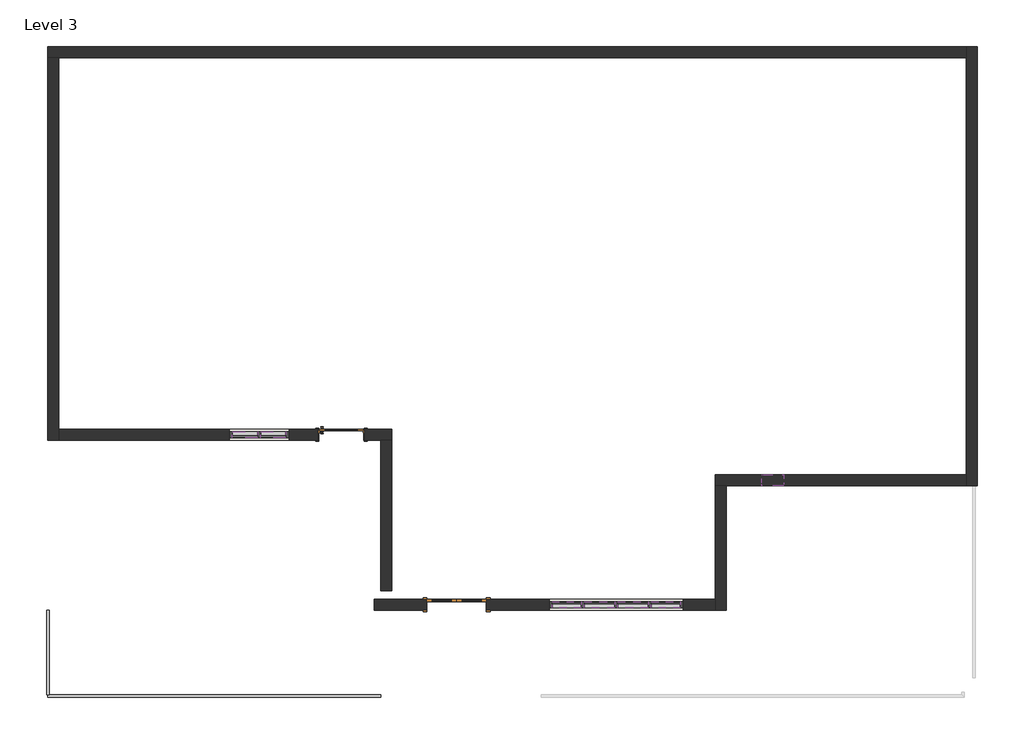
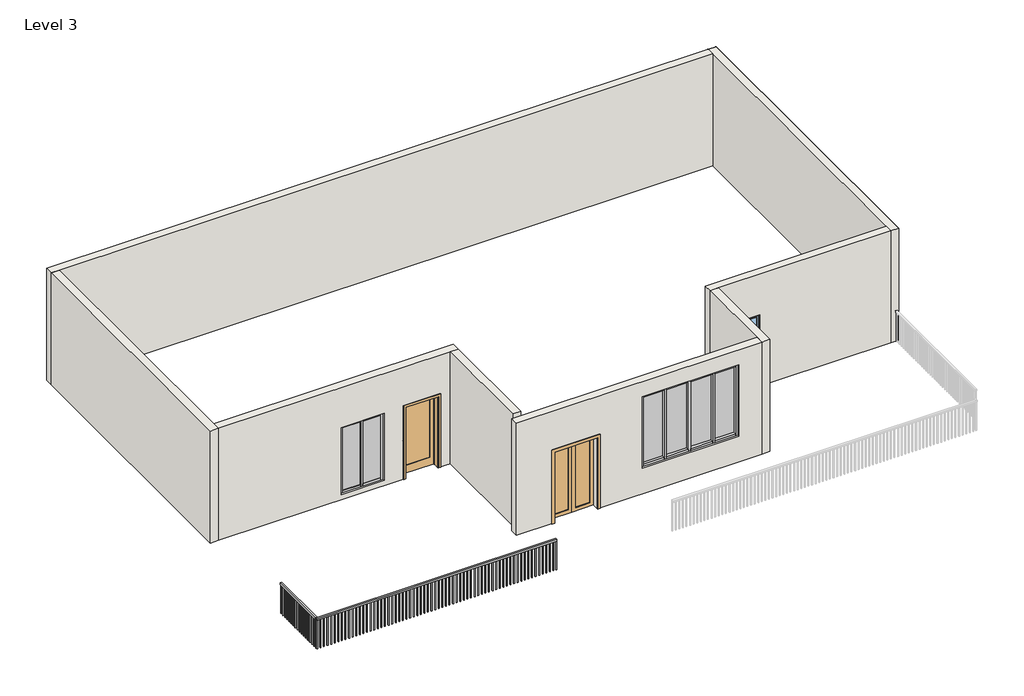
# One storey, part 1 of 2: 20 members, 8 walls, 6 plates, 2 doors, 2 railings, 1 window.
"""IFC4 building model written with IfcOpenShell, lengths in millimetres."""

from ifc_helpers import new_model, si_unit, frame, origin, place, context, project, spatial, polyline, outline, extrude, faceted_brep, transform, mapped, element, save
from components import door_double_glass_4_x_7_21e1f937, door_3b97b8e7, member_e5d39754, member_081e0693, member_3374d9b6, member_7cbddb58, member_0b7646a3, member_9d47184b, member_16b81337, system_panel_glazed_29c37de9, system_panel_glazed_550f7026, system_panel_glazed_af17b7d9, fixed_1_x1_542de505

model = new_model("IFC4")

# Units and contexts
model_context = context("Model", 3, world=origin())
ifc_project = project(units=[si_unit("LENGTHUNIT", "METRE", prefix="MILLI")], contexts=[model_context])

# Site, building, storey
site = spatial("IfcSite", under=ifc_project)
building = spatial("IfcBuilding", under=site)
storey = spatial("IfcBuildingStorey", under=building, Name="Level 3", Elevation=4114.8)

# Doors
placement = place(None, origin())
door_double_glass_4_x_7_shape = door_double_glass_4_x_7_21e1f937(model_context)
element("IfcDoor", 1, ObjectType="Door-Double-Glass : 4' x 7'", at=placement, inside=storey, context=model_context, shape_type="MappedRepresentation", body=[
    mapped(door_double_glass_4_x_7_shape, transform((-1827.2852284, -2816.9185169, 4114.8), x_axis=(1.0, 0.0, 0.0), y_axis=(0.0, 1.0, 0.0), z_axis=(0.0, 0.0, 1.0))),
])
door_shape = door_3b97b8e7(model_context)
element("IfcDoor", 2, ObjectType="Door-Interior-Single-1_Panel-Wood : 36\" x 84\"", at=placement, inside=storey, context=model_context, shape_type="MappedRepresentation", body=[
    mapped(door_shape, transform((-4180.3484006, 655.7377331, 4114.8), x_axis=(1.0, 0.0, 0.0), y_axis=(0.0, 1.0, 0.0), z_axis=(0.0, 0.0, 1.0))),
])

# Members
member_shape = member_e5d39754(model_context)
element("IfcMember", 3, ObjectType="Rectangular Mullion : 2.5\" x 5\" rectangular", at=placement, inside=storey, context=model_context, shape_type="MappedRepresentation", body=[
    mapped(member_shape, transform((2738.3647716, -2814.5372669, 7010.4), x_axis=(0.0, 0.0, 1.0), y_axis=(0.0, -1.0, 0.0), z_axis=(1.0, 0.0, 0.0))),
])
element("IfcMember", 4, ObjectType="Rectangular Mullion : 2.5\" x 5\" rectangular", at=placement, inside=storey, context=model_context, shape_type="MappedRepresentation", body=[
    mapped(member_shape, transform((712.7147716, -2814.5372669, 7010.4), x_axis=(0.0, 0.0, 1.0), y_axis=(0.0, -1.0, 0.0), z_axis=(1.0, 0.0, 0.0))),
])
element("IfcMember", 5, ObjectType="Rectangular Mullion : 2.5\" x 5\" rectangular", at=placement, inside=storey, context=model_context, shape_type="MappedRepresentation", body=[
    mapped(member_shape, transform((122.1647716, -2814.5372669, 4876.8), x_axis=(0.0, 0.0, -1.0), y_axis=(0.0, -1.0, 0.0), z_axis=(-1.0, 0.0, 0.0))),
])
element("IfcMember", 6, ObjectType="Rectangular Mullion : 2.5\" x 5\" rectangular", at=placement, inside=storey, context=model_context, shape_type="MappedRepresentation", body=[
    mapped(member_shape, transform((2147.8147716, -2814.5372669, 4876.8), x_axis=(0.0, 0.0, -1.0), y_axis=(0.0, -1.0, 0.0), z_axis=(-1.0, 0.0, 0.0))),
])
member_2_shape = member_081e0693(model_context)
element("IfcMember", 7, ObjectType="Rectangular Mullion : 2.5\" x 5\" rectangular", at=placement, inside=storey, context=model_context, shape_type="MappedRepresentation", body=[
    mapped(member_2_shape, transform((776.2147716, -2814.5372669, 4876.8), x_axis=(0.0, 0.0, -1.0), y_axis=(0.0, -1.0, 0.0), z_axis=(-1.0, 0.0, 0.0))),
])
element("IfcMember", 8, ObjectType="Rectangular Mullion : 2.5\" x 5\" rectangular", at=placement, inside=storey, context=model_context, shape_type="MappedRepresentation", body=[
    mapped(member_2_shape, transform((1462.0147716, -2814.5372669, 4876.8), x_axis=(0.0, 0.0, -1.0), y_axis=(0.0, -1.0, 0.0), z_axis=(-1.0, 0.0, 0.0))),
])
element("IfcMember", 9, ObjectType="Rectangular Mullion : 2.5\" x 5\" rectangular", at=placement, inside=storey, context=model_context, shape_type="MappedRepresentation", body=[
    mapped(member_2_shape, transform((1398.5147716, -2814.5372669, 7010.4), x_axis=(0.0, 0.0, 1.0), y_axis=(0.0, -1.0, 0.0), z_axis=(1.0, 0.0, 0.0))),
])
element("IfcMember", 10, ObjectType="Rectangular Mullion : 2.5\" x 5\" rectangular", at=placement, inside=storey, context=model_context, shape_type="MappedRepresentation", body=[
    mapped(member_2_shape, transform((2084.3147716, -2814.5372669, 7010.4), x_axis=(0.0, 0.0, 1.0), y_axis=(0.0, -1.0, 0.0), z_axis=(1.0, 0.0, 0.0))),
])
member_3_shape = member_3374d9b6(model_context)
element("IfcMember", 11, ObjectType="Rectangular Mullion : 2.5\" x 5\" rectangular", at=placement, inside=storey, context=model_context, shape_type="MappedRepresentation", body=[
    mapped(member_3_shape, transform((58.6647716, -2814.5372669, 7010.4), x_axis=(-1.0, 0.0, 0.0), y_axis=(0.0, -1.0, 0.0), z_axis=(0.0, 0.0, 1.0))),
])
element("IfcMember", 12, ObjectType="Rectangular Mullion : 2.5\" x 5\" rectangular", at=placement, inside=storey, context=model_context, shape_type="MappedRepresentation", body=[
    mapped(member_3_shape, transform((2801.8647716, -2814.5372669, 4876.8), x_axis=(1.0, 0.0, 0.0), y_axis=(0.0, -1.0, 0.0), z_axis=(0.0, 0.0, -1.0))),
])
member_4_shape = member_7cbddb58(model_context)
element("IfcMember", 13, ObjectType="Rectangular Mullion : 2.5\" x 5\" rectangular", at=placement, inside=storey, context=model_context, shape_type="MappedRepresentation", body=[
    mapped(member_4_shape, transform((744.4647716, -2814.5372669, 4876.8), x_axis=(1.0, 0.0, 0.0), y_axis=(0.0, -1.0, 0.0), z_axis=(0.0, 0.0, -1.0))),
])
element("IfcMember", 14, ObjectType="Rectangular Mullion : 2.5\" x 5\" rectangular", at=placement, inside=storey, context=model_context, shape_type="MappedRepresentation", body=[
    mapped(member_4_shape, transform((1430.2647716, -2814.5372669, 4876.8), x_axis=(1.0, 0.0, 0.0), y_axis=(0.0, -1.0, 0.0), z_axis=(0.0, 0.0, -1.0))),
])
element("IfcMember", 15, ObjectType="Rectangular Mullion : 2.5\" x 5\" rectangular", at=placement, inside=storey, context=model_context, shape_type="MappedRepresentation", body=[
    mapped(member_4_shape, transform((2116.0647716, -2814.5372669, 4876.8), x_axis=(1.0, 0.0, 0.0), y_axis=(0.0, -1.0, 0.0), z_axis=(0.0, 0.0, -1.0))),
])
member_5_shape = member_0b7646a3(model_context)
element("IfcMember", 16, ObjectType="Rectangular Mullion : 2.5\" x 5\" rectangular", at=placement, inside=storey, context=model_context, shape_type="MappedRepresentation", body=[
    mapped(member_5_shape, transform((-6402.8484006, 652.5627331, 6273.8), x_axis=(0.0, 0.0, 1.0), y_axis=(0.0, 1.0, 0.0), z_axis=(-1.0, 0.0, 0.0))),
])
element("IfcMember", 17, ObjectType="Rectangular Mullion : 2.5\" x 5\" rectangular", at=placement, inside=storey, context=model_context, shape_type="MappedRepresentation", body=[
    mapped(member_5_shape, transform((-5824.9984006, 652.5627331, 6273.8), x_axis=(0.0, 0.0, 1.0), y_axis=(0.0, 1.0, 0.0), z_axis=(-1.0, 0.0, 0.0))),
])
element("IfcMember", 18, ObjectType="Rectangular Mullion : 2.5\" x 5\" rectangular", at=placement, inside=storey, context=model_context, shape_type="MappedRepresentation", body=[
    mapped(member_5_shape, transform((-5310.6484006, 652.5627331, 4267.2), x_axis=(0.0, 0.0, -1.0), y_axis=(0.0, 1.0, 0.0), z_axis=(1.0, 0.0, 0.0))),
])
element("IfcMember", 19, ObjectType="Rectangular Mullion : 2.5\" x 5\" rectangular", at=placement, inside=storey, context=model_context, shape_type="MappedRepresentation", body=[
    mapped(member_5_shape, transform((-5888.4984006, 652.5627331, 4267.2), x_axis=(0.0, 0.0, -1.0), y_axis=(0.0, 1.0, 0.0), z_axis=(1.0, 0.0, 0.0))),
])
member_6_shape = member_9d47184b(model_context)
element("IfcMember", 20, ObjectType="Rectangular Mullion : 2.5\" x 5\" rectangular", at=placement, inside=storey, context=model_context, shape_type="MappedRepresentation", body=[
    mapped(member_6_shape, transform((-5856.7484006, 652.5627331, 4267.2), x_axis=(-1.0, 0.0, 0.0), y_axis=(0.0, 1.0, 0.0), z_axis=(0.0, 0.0, -1.0))),
])
member_7_shape = member_16b81337(model_context)
element("IfcMember", 21, ObjectType="Rectangular Mullion : 2.5\" x 5\" rectangular", at=placement, inside=storey, context=model_context, shape_type="MappedRepresentation", body=[
    mapped(member_7_shape, transform((-5247.1484006, 652.5627331, 6273.8), x_axis=(1.0, 0.0, 0.0), y_axis=(0.0, 1.0, 0.0), z_axis=(0.0, 0.0, 1.0))),
])
element("IfcMember", 22, ObjectType="Rectangular Mullion : 2.5\" x 5\" rectangular", at=placement, inside=storey, context=model_context, shape_type="MappedRepresentation", body=[
    mapped(member_7_shape, transform((-6466.3484006, 652.5627331, 4267.2), x_axis=(-1.0, 0.0, 0.0), y_axis=(0.0, 1.0, 0.0), z_axis=(0.0, 0.0, -1.0))),
])

# Plates
system_panel_glazed_shape = system_panel_glazed_29c37de9(model_context)
element("IfcPlate", 23, ObjectType="System Panel : Glazed", at=placement, inside=storey, context=model_context, shape_type="MappedRepresentation", body=[
    mapped(system_panel_glazed_shape, transform((417.4397716, -2814.5372669, 4940.3), x_axis=(1.0, 0.0, 0.0), y_axis=(0.0, 1.0, 0.0), z_axis=(0.0, 0.0, 1.0))),
])
element("IfcPlate", 24, ObjectType="System Panel : Glazed", at=placement, inside=storey, context=model_context, shape_type="MappedRepresentation", body=[
    mapped(system_panel_glazed_shape, transform((2443.0897716, -2814.5372669, 4940.3), x_axis=(1.0, 0.0, 0.0), y_axis=(0.0, 1.0, 0.0), z_axis=(0.0, 0.0, 1.0))),
])
system_panel_glazed_2_shape = system_panel_glazed_550f7026(model_context)
element("IfcPlate", 25, ObjectType="System Panel : Glazed", at=placement, inside=storey, context=model_context, shape_type="MappedRepresentation", body=[
    mapped(system_panel_glazed_2_shape, transform((1087.3647716, -2814.5372669, 4940.3), x_axis=(1.0, 0.0, 0.0), y_axis=(0.0, 1.0, 0.0), z_axis=(0.0, 0.0, 1.0))),
])
element("IfcPlate", 26, ObjectType="System Panel : Glazed", at=placement, inside=storey, context=model_context, shape_type="MappedRepresentation", body=[
    mapped(system_panel_glazed_2_shape, transform((1773.1647716, -2814.5372669, 4940.3), x_axis=(1.0, 0.0, 0.0), y_axis=(0.0, 1.0, 0.0), z_axis=(0.0, 0.0, 1.0))),
])
system_panel_glazed_3_shape = system_panel_glazed_af17b7d9(model_context)
element("IfcPlate", 27, ObjectType="System Panel : Glazed", at=placement, inside=storey, context=model_context, shape_type="MappedRepresentation", body=[
    mapped(system_panel_glazed_3_shape, transform((-5567.8234006, 652.5627331, 4330.7), x_axis=(-1.0, 0.0, 0.0), y_axis=(0.0, -1.0, 0.0), z_axis=(0.0, 0.0, 1.0))),
])
element("IfcPlate", 28, ObjectType="System Panel : Glazed", at=placement, inside=storey, context=model_context, shape_type="MappedRepresentation", body=[
    mapped(system_panel_glazed_3_shape, transform((-6145.6734006, 652.5627331, 4330.7), x_axis=(-1.0, 0.0, 0.0), y_axis=(0.0, -1.0, 0.0), z_axis=(0.0, 0.0, 1.0))),
])

# Railings
element("IfcRailing", 29, ObjectType="Handrail - Rectangular", at=placement, inside=storey, context=model_context, shape_type="SweptSolid", body=[
    extrude(outline(polyline([(-10171.1852284, -4706.8372669), (-10171.1852284, -4656.0372669), (-3380.2484006, -4656.0372669), (-3380.2484006, -4706.8372669), (-10171.1852284, -4706.8372669)])), frame((0.0, 0.0, 4978.4), z_axis=(0.0, 0.0, 1.0), x_axis=(1.0, 0.0, 0.0)), (0.0, 0.0, 1.0), 50.8),
    extrude(outline(polyline([(-3475.1102284, -4690.9622669), (-3475.1102284, -4671.9122669), (-3456.0602284, -4671.9122669), (-3456.0602284, -4690.9622669), (-3475.1102284, -4690.9622669)])), frame((0.0, 0.0, 4114.8), z_axis=(0.0, 0.0, 1.0), x_axis=(1.0, 0.0, 0.0)), (0.0, 0.0, 1.0), 863.6),
    extrude(outline(polyline([(-3576.7102284, -4690.9622669), (-3576.7102284, -4671.9122669), (-3557.6602284, -4671.9122669), (-3557.6602284, -4690.9622669), (-3576.7102284, -4690.9622669)])), frame((0.0, 0.0, 4114.8), z_axis=(0.0, 0.0, 1.0), x_axis=(1.0, 0.0, 0.0)), (0.0, 0.0, 1.0), 863.6),
    extrude(outline(polyline([(-3678.3102284, -4690.9622669), (-3678.3102284, -4671.9122669), (-3659.2602284, -4671.9122669), (-3659.2602284, -4690.9622669), (-3678.3102284, -4690.9622669)])), frame((0.0, 0.0, 4114.8), z_axis=(0.0, 0.0, 1.0), x_axis=(1.0, 0.0, 0.0)), (0.0, 0.0, 1.0), 863.6),
    extrude(outline(polyline([(-3779.9102284, -4690.9622669), (-3779.9102284, -4671.9122669), (-3760.8602284, -4671.9122669), (-3760.8602284, -4690.9622669), (-3779.9102284, -4690.9622669)])), frame((0.0, 0.0, 4114.8), z_axis=(0.0, 0.0, 1.0), x_axis=(1.0, 0.0, 0.0)), (0.0, 0.0, 1.0), 863.6),
    extrude(outline(polyline([(-3881.5102284, -4690.9622669), (-3881.5102284, -4671.9122669), (-3862.4602284, -4671.9122669), (-3862.4602284, -4690.9622669), (-3881.5102284, -4690.9622669)])), frame((0.0, 0.0, 4114.8), z_axis=(0.0, 0.0, 1.0), x_axis=(1.0, 0.0, 0.0)), (0.0, 0.0, 1.0), 863.6),
    extrude(outline(polyline([(-3983.1102284, -4690.9622669), (-3983.1102284, -4671.9122669), (-3964.0602284, -4671.9122669), (-3964.0602284, -4690.9622669), (-3983.1102284, -4690.9622669)])), frame((0.0, 0.0, 4114.8), z_axis=(0.0, 0.0, 1.0), x_axis=(1.0, 0.0, 0.0)), (0.0, 0.0, 1.0), 863.6),
    extrude(outline(polyline([(-4084.7102284, -4690.9622669), (-4084.7102284, -4671.9122669), (-4065.6602284, -4671.9122669), (-4065.6602284, -4690.9622669), (-4084.7102284, -4690.9622669)])), frame((0.0, 0.0, 4114.8), z_axis=(0.0, 0.0, 1.0), x_axis=(1.0, 0.0, 0.0)), (0.0, 0.0, 1.0), 863.6),
    extrude(outline(polyline([(-4186.3102284, -4690.9622669), (-4186.3102284, -4671.9122669), (-4167.2602284, -4671.9122669), (-4167.2602284, -4690.9622669), (-4186.3102284, -4690.9622669)])), frame((0.0, 0.0, 4114.8), z_axis=(0.0, 0.0, 1.0), x_axis=(1.0, 0.0, 0.0)), (0.0, 0.0, 1.0), 863.6),
    extrude(outline(polyline([(-4287.9102284, -4690.9622669), (-4287.9102284, -4671.9122669), (-4268.8602284, -4671.9122669), (-4268.8602284, -4690.9622669), (-4287.9102284, -4690.9622669)])), frame((0.0, 0.0, 4114.8), z_axis=(0.0, 0.0, 1.0), x_axis=(1.0, 0.0, 0.0)), (0.0, 0.0, 1.0), 863.6),
    extrude(outline(polyline([(-4389.5102284, -4690.9622669), (-4389.5102284, -4671.9122669), (-4370.4602284, -4671.9122669), (-4370.4602284, -4690.9622669), (-4389.5102284, -4690.9622669)])), frame((0.0, 0.0, 4114.8), z_axis=(0.0, 0.0, 1.0), x_axis=(1.0, 0.0, 0.0)), (0.0, 0.0, 1.0), 863.6),
    extrude(outline(polyline([(-4491.1102284, -4690.9622669), (-4491.1102284, -4671.9122669), (-4472.0602284, -4671.9122669), (-4472.0602284, -4690.9622669), (-4491.1102284, -4690.9622669)])), frame((0.0, 0.0, 4114.8), z_axis=(0.0, 0.0, 1.0), x_axis=(1.0, 0.0, 0.0)), (0.0, 0.0, 1.0), 863.6),
    extrude(outline(polyline([(-4592.7102284, -4690.9622669), (-4592.7102284, -4671.9122669), (-4573.6602284, -4671.9122669), (-4573.6602284, -4690.9622669), (-4592.7102284, -4690.9622669)])), frame((0.0, 0.0, 4114.8), z_axis=(0.0, 0.0, 1.0), x_axis=(1.0, 0.0, 0.0)), (0.0, 0.0, 1.0), 863.6),
    extrude(outline(polyline([(-4694.3102284, -4690.9622669), (-4694.3102284, -4671.9122669), (-4675.2602284, -4671.9122669), (-4675.2602284, -4690.9622669), (-4694.3102284, -4690.9622669)])), frame((0.0, 0.0, 4114.8), z_axis=(0.0, 0.0, 1.0), x_axis=(1.0, 0.0, 0.0)), (0.0, 0.0, 1.0), 863.6),
    extrude(outline(polyline([(-4795.9102284, -4690.9622669), (-4795.9102284, -4671.9122669), (-4776.8602284, -4671.9122669), (-4776.8602284, -4690.9622669), (-4795.9102284, -4690.9622669)])), frame((0.0, 0.0, 4114.8), z_axis=(0.0, 0.0, 1.0), x_axis=(1.0, 0.0, 0.0)), (0.0, 0.0, 1.0), 863.6),
    extrude(outline(polyline([(-4897.5102284, -4690.9622669), (-4897.5102284, -4671.9122669), (-4878.4602284, -4671.9122669), (-4878.4602284, -4690.9622669), (-4897.5102284, -4690.9622669)])), frame((0.0, 0.0, 4114.8), z_axis=(0.0, 0.0, 1.0), x_axis=(1.0, 0.0, 0.0)), (0.0, 0.0, 1.0), 863.6),
    extrude(outline(polyline([(-4999.1102284, -4690.9622669), (-4999.1102284, -4671.9122669), (-4980.0602284, -4671.9122669), (-4980.0602284, -4690.9622669), (-4999.1102284, -4690.9622669)])), frame((0.0, 0.0, 4114.8), z_axis=(0.0, 0.0, 1.0), x_axis=(1.0, 0.0, 0.0)), (0.0, 0.0, 1.0), 863.6),
    extrude(outline(polyline([(-5100.7102284, -4690.9622669), (-5100.7102284, -4671.9122669), (-5081.6602284, -4671.9122669), (-5081.6602284, -4690.9622669), (-5100.7102284, -4690.9622669)])), frame((0.0, 0.0, 4114.8), z_axis=(0.0, 0.0, 1.0), x_axis=(1.0, 0.0, 0.0)), (0.0, 0.0, 1.0), 863.6),
    extrude(outline(polyline([(-5202.3102284, -4690.9622669), (-5202.3102284, -4671.9122669), (-5183.2602284, -4671.9122669), (-5183.2602284, -4690.9622669), (-5202.3102284, -4690.9622669)])), frame((0.0, 0.0, 4114.8), z_axis=(0.0, 0.0, 1.0), x_axis=(1.0, 0.0, 0.0)), (0.0, 0.0, 1.0), 863.6),
    extrude(outline(polyline([(-5303.9102284, -4690.9622669), (-5303.9102284, -4671.9122669), (-5284.8602284, -4671.9122669), (-5284.8602284, -4690.9622669), (-5303.9102284, -4690.9622669)])), frame((0.0, 0.0, 4114.8), z_axis=(0.0, 0.0, 1.0), x_axis=(1.0, 0.0, 0.0)), (0.0, 0.0, 1.0), 863.6),
    extrude(outline(polyline([(-5405.5102284, -4690.9622669), (-5405.5102284, -4671.9122669), (-5386.4602284, -4671.9122669), (-5386.4602284, -4690.9622669), (-5405.5102284, -4690.9622669)])), frame((0.0, 0.0, 4114.8), z_axis=(0.0, 0.0, 1.0), x_axis=(1.0, 0.0, 0.0)), (0.0, 0.0, 1.0), 863.6),
    extrude(outline(polyline([(-5507.1102284, -4690.9622669), (-5507.1102284, -4671.9122669), (-5488.0602284, -4671.9122669), (-5488.0602284, -4690.9622669), (-5507.1102284, -4690.9622669)])), frame((0.0, 0.0, 4114.8), z_axis=(0.0, 0.0, 1.0), x_axis=(1.0, 0.0, 0.0)), (0.0, 0.0, 1.0), 863.6),
    extrude(outline(polyline([(-5608.7102284, -4690.9622669), (-5608.7102284, -4671.9122669), (-5589.6602284, -4671.9122669), (-5589.6602284, -4690.9622669), (-5608.7102284, -4690.9622669)])), frame((0.0, 0.0, 4114.8), z_axis=(0.0, 0.0, 1.0), x_axis=(1.0, 0.0, 0.0)), (0.0, 0.0, 1.0), 863.6),
    extrude(outline(polyline([(-5710.3102284, -4690.9622669), (-5710.3102284, -4671.9122669), (-5691.2602284, -4671.9122669), (-5691.2602284, -4690.9622669), (-5710.3102284, -4690.9622669)])), frame((0.0, 0.0, 4114.8), z_axis=(0.0, 0.0, 1.0), x_axis=(1.0, 0.0, 0.0)), (0.0, 0.0, 1.0), 863.6),
    extrude(outline(polyline([(-5811.9102284, -4690.9622669), (-5811.9102284, -4671.9122669), (-5792.8602284, -4671.9122669), (-5792.8602284, -4690.9622669), (-5811.9102284, -4690.9622669)])), frame((0.0, 0.0, 4114.8), z_axis=(0.0, 0.0, 1.0), x_axis=(1.0, 0.0, 0.0)), (0.0, 0.0, 1.0), 863.6),
    extrude(outline(polyline([(-5913.5102284, -4690.9622669), (-5913.5102284, -4671.9122669), (-5894.4602284, -4671.9122669), (-5894.4602284, -4690.9622669), (-5913.5102284, -4690.9622669)])), frame((0.0, 0.0, 4114.8), z_axis=(0.0, 0.0, 1.0), x_axis=(1.0, 0.0, 0.0)), (0.0, 0.0, 1.0), 863.6),
    extrude(outline(polyline([(-6015.1102284, -4690.9622669), (-6015.1102284, -4671.9122669), (-5996.0602284, -4671.9122669), (-5996.0602284, -4690.9622669), (-6015.1102284, -4690.9622669)])), frame((0.0, 0.0, 4114.8), z_axis=(0.0, 0.0, 1.0), x_axis=(1.0, 0.0, 0.0)), (0.0, 0.0, 1.0), 863.6),
    extrude(outline(polyline([(-6116.7102284, -4690.9622669), (-6116.7102284, -4671.9122669), (-6097.6602284, -4671.9122669), (-6097.6602284, -4690.9622669), (-6116.7102284, -4690.9622669)])), frame((0.0, 0.0, 4114.8), z_axis=(0.0, 0.0, 1.0), x_axis=(1.0, 0.0, 0.0)), (0.0, 0.0, 1.0), 863.6),
    extrude(outline(polyline([(-6218.3102284, -4690.9622669), (-6218.3102284, -4671.9122669), (-6199.2602284, -4671.9122669), (-6199.2602284, -4690.9622669), (-6218.3102284, -4690.9622669)])), frame((0.0, 0.0, 4114.8), z_axis=(0.0, 0.0, 1.0), x_axis=(1.0, 0.0, 0.0)), (0.0, 0.0, 1.0), 863.6),
    extrude(outline(polyline([(-6319.9102284, -4690.9622669), (-6319.9102284, -4671.9122669), (-6300.8602284, -4671.9122669), (-6300.8602284, -4690.9622669), (-6319.9102284, -4690.9622669)])), frame((0.0, 0.0, 4114.8), z_axis=(0.0, 0.0, 1.0), x_axis=(1.0, 0.0, 0.0)), (0.0, 0.0, 1.0), 863.6),
    extrude(outline(polyline([(-6421.5102284, -4690.9622669), (-6421.5102284, -4671.9122669), (-6402.4602284, -4671.9122669), (-6402.4602284, -4690.9622669), (-6421.5102284, -4690.9622669)])), frame((0.0, 0.0, 4114.8), z_axis=(0.0, 0.0, 1.0), x_axis=(1.0, 0.0, 0.0)), (0.0, 0.0, 1.0), 863.6),
    extrude(outline(polyline([(-6523.1102284, -4690.9622669), (-6523.1102284, -4671.9122669), (-6504.0602284, -4671.9122669), (-6504.0602284, -4690.9622669), (-6523.1102284, -4690.9622669)])), frame((0.0, 0.0, 4114.8), z_axis=(0.0, 0.0, 1.0), x_axis=(1.0, 0.0, 0.0)), (0.0, 0.0, 1.0), 863.6),
    extrude(outline(polyline([(-6624.7102284, -4690.9622669), (-6624.7102284, -4671.9122669), (-6605.6602284, -4671.9122669), (-6605.6602284, -4690.9622669), (-6624.7102284, -4690.9622669)])), frame((0.0, 0.0, 4114.8), z_axis=(0.0, 0.0, 1.0), x_axis=(1.0, 0.0, 0.0)), (0.0, 0.0, 1.0), 863.6),
    extrude(outline(polyline([(-6726.3102284, -4690.9622669), (-6726.3102284, -4671.9122669), (-6707.2602284, -4671.9122669), (-6707.2602284, -4690.9622669), (-6726.3102284, -4690.9622669)])), frame((0.0, 0.0, 4114.8), z_axis=(0.0, 0.0, 1.0), x_axis=(1.0, 0.0, 0.0)), (0.0, 0.0, 1.0), 863.6),
    extrude(outline(polyline([(-6827.9102284, -4690.9622669), (-6827.9102284, -4671.9122669), (-6808.8602284, -4671.9122669), (-6808.8602284, -4690.9622669), (-6827.9102284, -4690.9622669)])), frame((0.0, 0.0, 4114.8), z_axis=(0.0, 0.0, 1.0), x_axis=(1.0, 0.0, 0.0)), (0.0, 0.0, 1.0), 863.6),
    extrude(outline(polyline([(-6929.5102284, -4690.9622669), (-6929.5102284, -4671.9122669), (-6910.4602284, -4671.9122669), (-6910.4602284, -4690.9622669), (-6929.5102284, -4690.9622669)])), frame((0.0, 0.0, 4114.8), z_axis=(0.0, 0.0, 1.0), x_axis=(1.0, 0.0, 0.0)), (0.0, 0.0, 1.0), 863.6),
    extrude(outline(polyline([(-7031.1102284, -4690.9622669), (-7031.1102284, -4671.9122669), (-7012.0602284, -4671.9122669), (-7012.0602284, -4690.9622669), (-7031.1102284, -4690.9622669)])), frame((0.0, 0.0, 4114.8), z_axis=(0.0, 0.0, 1.0), x_axis=(1.0, 0.0, 0.0)), (0.0, 0.0, 1.0), 863.6),
    extrude(outline(polyline([(-7132.7102284, -4690.9622669), (-7132.7102284, -4671.9122669), (-7113.6602284, -4671.9122669), (-7113.6602284, -4690.9622669), (-7132.7102284, -4690.9622669)])), frame((0.0, 0.0, 4114.8), z_axis=(0.0, 0.0, 1.0), x_axis=(1.0, 0.0, 0.0)), (0.0, 0.0, 1.0), 863.6),
    extrude(outline(polyline([(-7234.3102284, -4690.9622669), (-7234.3102284, -4671.9122669), (-7215.2602284, -4671.9122669), (-7215.2602284, -4690.9622669), (-7234.3102284, -4690.9622669)])), frame((0.0, 0.0, 4114.8), z_axis=(0.0, 0.0, 1.0), x_axis=(1.0, 0.0, 0.0)), (0.0, 0.0, 1.0), 863.6),
    extrude(outline(polyline([(-7335.9102284, -4690.9622669), (-7335.9102284, -4671.9122669), (-7316.8602284, -4671.9122669), (-7316.8602284, -4690.9622669), (-7335.9102284, -4690.9622669)])), frame((0.0, 0.0, 4114.8), z_axis=(0.0, 0.0, 1.0), x_axis=(1.0, 0.0, 0.0)), (0.0, 0.0, 1.0), 863.6),
    extrude(outline(polyline([(-7437.5102284, -4690.9622669), (-7437.5102284, -4671.9122669), (-7418.4602284, -4671.9122669), (-7418.4602284, -4690.9622669), (-7437.5102284, -4690.9622669)])), frame((0.0, 0.0, 4114.8), z_axis=(0.0, 0.0, 1.0), x_axis=(1.0, 0.0, 0.0)), (0.0, 0.0, 1.0), 863.6),
    extrude(outline(polyline([(-7539.1102284, -4690.9622669), (-7539.1102284, -4671.9122669), (-7520.0602284, -4671.9122669), (-7520.0602284, -4690.9622669), (-7539.1102284, -4690.9622669)])), frame((0.0, 0.0, 4114.8), z_axis=(0.0, 0.0, 1.0), x_axis=(1.0, 0.0, 0.0)), (0.0, 0.0, 1.0), 863.6),
    extrude(outline(polyline([(-7640.7102284, -4690.9622669), (-7640.7102284, -4671.9122669), (-7621.6602284, -4671.9122669), (-7621.6602284, -4690.9622669), (-7640.7102284, -4690.9622669)])), frame((0.0, 0.0, 4114.8), z_axis=(0.0, 0.0, 1.0), x_axis=(1.0, 0.0, 0.0)), (0.0, 0.0, 1.0), 863.6),
    extrude(outline(polyline([(-7742.3102284, -4690.9622669), (-7742.3102284, -4671.9122669), (-7723.2602284, -4671.9122669), (-7723.2602284, -4690.9622669), (-7742.3102284, -4690.9622669)])), frame((0.0, 0.0, 4114.8), z_axis=(0.0, 0.0, 1.0), x_axis=(1.0, 0.0, 0.0)), (0.0, 0.0, 1.0), 863.6),
    extrude(outline(polyline([(-7843.9102284, -4690.9622669), (-7843.9102284, -4671.9122669), (-7824.8602284, -4671.9122669), (-7824.8602284, -4690.9622669), (-7843.9102284, -4690.9622669)])), frame((0.0, 0.0, 4114.8), z_axis=(0.0, 0.0, 1.0), x_axis=(1.0, 0.0, 0.0)), (0.0, 0.0, 1.0), 863.6),
    extrude(outline(polyline([(-7945.5102284, -4690.9622669), (-7945.5102284, -4671.9122669), (-7926.4602284, -4671.9122669), (-7926.4602284, -4690.9622669), (-7945.5102284, -4690.9622669)])), frame((0.0, 0.0, 4114.8), z_axis=(0.0, 0.0, 1.0), x_axis=(1.0, 0.0, 0.0)), (0.0, 0.0, 1.0), 863.6),
    extrude(outline(polyline([(-8047.1102284, -4690.9622669), (-8047.1102284, -4671.9122669), (-8028.0602284, -4671.9122669), (-8028.0602284, -4690.9622669), (-8047.1102284, -4690.9622669)])), frame((0.0, 0.0, 4114.8), z_axis=(0.0, 0.0, 1.0), x_axis=(1.0, 0.0, 0.0)), (0.0, 0.0, 1.0), 863.6),
    extrude(outline(polyline([(-8148.7102284, -4690.9622669), (-8148.7102284, -4671.9122669), (-8129.6602284, -4671.9122669), (-8129.6602284, -4690.9622669), (-8148.7102284, -4690.9622669)])), frame((0.0, 0.0, 4114.8), z_axis=(0.0, 0.0, 1.0), x_axis=(1.0, 0.0, 0.0)), (0.0, 0.0, 1.0), 863.6),
    extrude(outline(polyline([(-8250.3102284, -4690.9622669), (-8250.3102284, -4671.9122669), (-8231.2602284, -4671.9122669), (-8231.2602284, -4690.9622669), (-8250.3102284, -4690.9622669)])), frame((0.0, 0.0, 4114.8), z_axis=(0.0, 0.0, 1.0), x_axis=(1.0, 0.0, 0.0)), (0.0, 0.0, 1.0), 863.6),
    extrude(outline(polyline([(-8351.9102284, -4690.9622669), (-8351.9102284, -4671.9122669), (-8332.8602284, -4671.9122669), (-8332.8602284, -4690.9622669), (-8351.9102284, -4690.9622669)])), frame((0.0, 0.0, 4114.8), z_axis=(0.0, 0.0, 1.0), x_axis=(1.0, 0.0, 0.0)), (0.0, 0.0, 1.0), 863.6),
    extrude(outline(polyline([(-8453.5102284, -4690.9622669), (-8453.5102284, -4671.9122669), (-8434.4602284, -4671.9122669), (-8434.4602284, -4690.9622669), (-8453.5102284, -4690.9622669)])), frame((0.0, 0.0, 4114.8), z_axis=(0.0, 0.0, 1.0), x_axis=(1.0, 0.0, 0.0)), (0.0, 0.0, 1.0), 863.6),
    extrude(outline(polyline([(-8555.1102284, -4690.9622669), (-8555.1102284, -4671.9122669), (-8536.0602284, -4671.9122669), (-8536.0602284, -4690.9622669), (-8555.1102284, -4690.9622669)])), frame((0.0, 0.0, 4114.8), z_axis=(0.0, 0.0, 1.0), x_axis=(1.0, 0.0, 0.0)), (0.0, 0.0, 1.0), 863.6),
    extrude(outline(polyline([(-8656.7102284, -4690.9622669), (-8656.7102284, -4671.9122669), (-8637.6602284, -4671.9122669), (-8637.6602284, -4690.9622669), (-8656.7102284, -4690.9622669)])), frame((0.0, 0.0, 4114.8), z_axis=(0.0, 0.0, 1.0), x_axis=(1.0, 0.0, 0.0)), (0.0, 0.0, 1.0), 863.6),
    extrude(outline(polyline([(-8758.3102284, -4690.9622669), (-8758.3102284, -4671.9122669), (-8739.2602284, -4671.9122669), (-8739.2602284, -4690.9622669), (-8758.3102284, -4690.9622669)])), frame((0.0, 0.0, 4114.8), z_axis=(0.0, 0.0, 1.0), x_axis=(1.0, 0.0, 0.0)), (0.0, 0.0, 1.0), 863.6),
    extrude(outline(polyline([(-8859.9102284, -4690.9622669), (-8859.9102284, -4671.9122669), (-8840.8602284, -4671.9122669), (-8840.8602284, -4690.9622669), (-8859.9102284, -4690.9622669)])), frame((0.0, 0.0, 4114.8), z_axis=(0.0, 0.0, 1.0), x_axis=(1.0, 0.0, 0.0)), (0.0, 0.0, 1.0), 863.6),
    extrude(outline(polyline([(-8961.5102284, -4690.9622669), (-8961.5102284, -4671.9122669), (-8942.4602284, -4671.9122669), (-8942.4602284, -4690.9622669), (-8961.5102284, -4690.9622669)])), frame((0.0, 0.0, 4114.8), z_axis=(0.0, 0.0, 1.0), x_axis=(1.0, 0.0, 0.0)), (0.0, 0.0, 1.0), 863.6),
    extrude(outline(polyline([(-9063.1102284, -4690.9622669), (-9063.1102284, -4671.9122669), (-9044.0602284, -4671.9122669), (-9044.0602284, -4690.9622669), (-9063.1102284, -4690.9622669)])), frame((0.0, 0.0, 4114.8), z_axis=(0.0, 0.0, 1.0), x_axis=(1.0, 0.0, 0.0)), (0.0, 0.0, 1.0), 863.6),
    extrude(outline(polyline([(-9164.7102284, -4690.9622669), (-9164.7102284, -4671.9122669), (-9145.6602284, -4671.9122669), (-9145.6602284, -4690.9622669), (-9164.7102284, -4690.9622669)])), frame((0.0, 0.0, 4114.8), z_axis=(0.0, 0.0, 1.0), x_axis=(1.0, 0.0, 0.0)), (0.0, 0.0, 1.0), 863.6),
    extrude(outline(polyline([(-9266.3102284, -4690.9622669), (-9266.3102284, -4671.9122669), (-9247.2602284, -4671.9122669), (-9247.2602284, -4690.9622669), (-9266.3102284, -4690.9622669)])), frame((0.0, 0.0, 4114.8), z_axis=(0.0, 0.0, 1.0), x_axis=(1.0, 0.0, 0.0)), (0.0, 0.0, 1.0), 863.6),
    extrude(outline(polyline([(-9367.9102284, -4690.9622669), (-9367.9102284, -4671.9122669), (-9348.8602284, -4671.9122669), (-9348.8602284, -4690.9622669), (-9367.9102284, -4690.9622669)])), frame((0.0, 0.0, 4114.8), z_axis=(0.0, 0.0, 1.0), x_axis=(1.0, 0.0, 0.0)), (0.0, 0.0, 1.0), 863.6),
    extrude(outline(polyline([(-9469.5102284, -4690.9622669), (-9469.5102284, -4671.9122669), (-9450.4602284, -4671.9122669), (-9450.4602284, -4690.9622669), (-9469.5102284, -4690.9622669)])), frame((0.0, 0.0, 4114.8), z_axis=(0.0, 0.0, 1.0), x_axis=(1.0, 0.0, 0.0)), (0.0, 0.0, 1.0), 863.6),
    extrude(outline(polyline([(-9571.1102284, -4690.9622669), (-9571.1102284, -4671.9122669), (-9552.0602284, -4671.9122669), (-9552.0602284, -4690.9622669), (-9571.1102284, -4690.9622669)])), frame((0.0, 0.0, 4114.8), z_axis=(0.0, 0.0, 1.0), x_axis=(1.0, 0.0, 0.0)), (0.0, 0.0, 1.0), 863.6),
    extrude(outline(polyline([(-9672.7102284, -4690.9622669), (-9672.7102284, -4671.9122669), (-9653.6602284, -4671.9122669), (-9653.6602284, -4690.9622669), (-9672.7102284, -4690.9622669)])), frame((0.0, 0.0, 4114.8), z_axis=(0.0, 0.0, 1.0), x_axis=(1.0, 0.0, 0.0)), (0.0, 0.0, 1.0), 863.6),
    extrude(outline(polyline([(-9774.3102284, -4690.9622669), (-9774.3102284, -4671.9122669), (-9755.2602284, -4671.9122669), (-9755.2602284, -4690.9622669), (-9774.3102284, -4690.9622669)])), frame((0.0, 0.0, 4114.8), z_axis=(0.0, 0.0, 1.0), x_axis=(1.0, 0.0, 0.0)), (0.0, 0.0, 1.0), 863.6),
    extrude(outline(polyline([(-9875.9102284, -4690.9622669), (-9875.9102284, -4671.9122669), (-9856.8602284, -4671.9122669), (-9856.8602284, -4690.9622669), (-9875.9102284, -4690.9622669)])), frame((0.0, 0.0, 4114.8), z_axis=(0.0, 0.0, 1.0), x_axis=(1.0, 0.0, 0.0)), (0.0, 0.0, 1.0), 863.6),
    extrude(outline(polyline([(-9977.5102284, -4690.9622669), (-9977.5102284, -4671.9122669), (-9958.4602284, -4671.9122669), (-9958.4602284, -4690.9622669), (-9977.5102284, -4690.9622669)])), frame((0.0, 0.0, 4114.8), z_axis=(0.0, 0.0, 1.0), x_axis=(1.0, 0.0, 0.0)), (0.0, 0.0, 1.0), 863.6),
    extrude(outline(polyline([(-10079.1102284, -4690.9622669), (-10079.1102284, -4671.9122669), (-10060.0602284, -4671.9122669), (-10060.0602284, -4690.9622669), (-10079.1102284, -4690.9622669)])), frame((0.0, 0.0, 4114.8), z_axis=(0.0, 0.0, 1.0), x_axis=(1.0, 0.0, 0.0)), (0.0, 0.0, 1.0), 863.6),
    extrude(outline(polyline([(-3399.2984006, -4690.9622669), (-3399.2984006, -4671.9122669), (-3380.2484006, -4671.9122669), (-3380.2484006, -4690.9622669), (-3399.2984006, -4690.9622669)])), frame((0.0, 0.0, 4114.8), z_axis=(0.0, 0.0, 1.0), x_axis=(1.0, 0.0, 0.0)), (0.0, 0.0, 1.0), 863.6),
    extrude(outline(polyline([(-10171.1852284, -4690.9622669), (-10171.1852284, -4671.9122669), (-10152.1352284, -4671.9122669), (-10152.1352284, -4690.9622669), (-10171.1852284, -4690.9622669)])), frame((0.0, 0.0, 4114.8), z_axis=(0.0, 0.0, 1.0), x_axis=(1.0, 0.0, 0.0)), (0.0, 0.0, 1.0), 863.6),
])
element("IfcRailing", 30, ObjectType="Handrail - Rectangular", at=placement, inside=storey, context=model_context, shape_type="SweptSolid", body=[
    extrude(outline(polyline([(-10145.7852284, -4656.0372669), (-10196.5852284, -4656.0372669), (-10196.5852284, -2928.8372669), (-10145.7852284, -2928.8372669), (-10145.7852284, -4656.0372669)])), frame((0.0, 0.0, 4978.4), z_axis=(0.0, 0.0, 1.0), x_axis=(1.0, 0.0, 0.0)), (0.0, 0.0, 1.0), 50.8),
    extrude(outline(polyline([(-10161.6602284, -3039.9622669), (-10180.7102284, -3039.9622669), (-10180.7102284, -3020.9122669), (-10161.6602284, -3020.9122669), (-10161.6602284, -3039.9622669)])), frame((0.0, 0.0, 4114.8), z_axis=(0.0, 0.0, 1.0), x_axis=(1.0, 0.0, 0.0)), (0.0, 0.0, 1.0), 863.6),
    extrude(outline(polyline([(-10161.6602284, -3141.5622669), (-10180.7102284, -3141.5622669), (-10180.7102284, -3122.5122669), (-10161.6602284, -3122.5122669), (-10161.6602284, -3141.5622669)])), frame((0.0, 0.0, 4114.8), z_axis=(0.0, 0.0, 1.0), x_axis=(1.0, 0.0, 0.0)), (0.0, 0.0, 1.0), 863.6),
    extrude(outline(polyline([(-10161.6602284, -3243.1622669), (-10180.7102284, -3243.1622669), (-10180.7102284, -3224.1122669), (-10161.6602284, -3224.1122669), (-10161.6602284, -3243.1622669)])), frame((0.0, 0.0, 4114.8), z_axis=(0.0, 0.0, 1.0), x_axis=(1.0, 0.0, 0.0)), (0.0, 0.0, 1.0), 863.6),
    extrude(outline(polyline([(-10161.6602284, -3344.7622669), (-10180.7102284, -3344.7622669), (-10180.7102284, -3325.7122669), (-10161.6602284, -3325.7122669), (-10161.6602284, -3344.7622669)])), frame((0.0, 0.0, 4114.8), z_axis=(0.0, 0.0, 1.0), x_axis=(1.0, 0.0, 0.0)), (0.0, 0.0, 1.0), 863.6),
    extrude(outline(polyline([(-10161.6602284, -3446.3622669), (-10180.7102284, -3446.3622669), (-10180.7102284, -3427.3122669), (-10161.6602284, -3427.3122669), (-10161.6602284, -3446.3622669)])), frame((0.0, 0.0, 4114.8), z_axis=(0.0, 0.0, 1.0), x_axis=(1.0, 0.0, 0.0)), (0.0, 0.0, 1.0), 863.6),
    extrude(outline(polyline([(-10161.6602284, -3547.9622669), (-10180.7102284, -3547.9622669), (-10180.7102284, -3528.9122669), (-10161.6602284, -3528.9122669), (-10161.6602284, -3547.9622669)])), frame((0.0, 0.0, 4114.8), z_axis=(0.0, 0.0, 1.0), x_axis=(1.0, 0.0, 0.0)), (0.0, 0.0, 1.0), 863.6),
    extrude(outline(polyline([(-10161.6602284, -3649.5622669), (-10180.7102284, -3649.5622669), (-10180.7102284, -3630.5122669), (-10161.6602284, -3630.5122669), (-10161.6602284, -3649.5622669)])), frame((0.0, 0.0, 4114.8), z_axis=(0.0, 0.0, 1.0), x_axis=(1.0, 0.0, 0.0)), (0.0, 0.0, 1.0), 863.6),
    extrude(outline(polyline([(-10161.6602284, -3751.1622669), (-10180.7102284, -3751.1622669), (-10180.7102284, -3732.1122669), (-10161.6602284, -3732.1122669), (-10161.6602284, -3751.1622669)])), frame((0.0, 0.0, 4114.8), z_axis=(0.0, 0.0, 1.0), x_axis=(1.0, 0.0, 0.0)), (0.0, 0.0, 1.0), 863.6),
    extrude(outline(polyline([(-10161.6602284, -3852.7622669), (-10180.7102284, -3852.7622669), (-10180.7102284, -3833.7122669), (-10161.6602284, -3833.7122669), (-10161.6602284, -3852.7622669)])), frame((0.0, 0.0, 4114.8), z_axis=(0.0, 0.0, 1.0), x_axis=(1.0, 0.0, 0.0)), (0.0, 0.0, 1.0), 863.6),
    extrude(outline(polyline([(-10161.6602284, -3954.3622669), (-10180.7102284, -3954.3622669), (-10180.7102284, -3935.3122669), (-10161.6602284, -3935.3122669), (-10161.6602284, -3954.3622669)])), frame((0.0, 0.0, 4114.8), z_axis=(0.0, 0.0, 1.0), x_axis=(1.0, 0.0, 0.0)), (0.0, 0.0, 1.0), 863.6),
    extrude(outline(polyline([(-10161.6602284, -4055.9622669), (-10180.7102284, -4055.9622669), (-10180.7102284, -4036.9122669), (-10161.6602284, -4036.9122669), (-10161.6602284, -4055.9622669)])), frame((0.0, 0.0, 4114.8), z_axis=(0.0, 0.0, 1.0), x_axis=(1.0, 0.0, 0.0)), (0.0, 0.0, 1.0), 863.6),
    extrude(outline(polyline([(-10161.6602284, -4157.5622669), (-10180.7102284, -4157.5622669), (-10180.7102284, -4138.5122669), (-10161.6602284, -4138.5122669), (-10161.6602284, -4157.5622669)])), frame((0.0, 0.0, 4114.8), z_axis=(0.0, 0.0, 1.0), x_axis=(1.0, 0.0, 0.0)), (0.0, 0.0, 1.0), 863.6),
    extrude(outline(polyline([(-10161.6602284, -4259.1622669), (-10180.7102284, -4259.1622669), (-10180.7102284, -4240.1122669), (-10161.6602284, -4240.1122669), (-10161.6602284, -4259.1622669)])), frame((0.0, 0.0, 4114.8), z_axis=(0.0, 0.0, 1.0), x_axis=(1.0, 0.0, 0.0)), (0.0, 0.0, 1.0), 863.6),
    extrude(outline(polyline([(-10161.6602284, -4360.7622669), (-10180.7102284, -4360.7622669), (-10180.7102284, -4341.7122669), (-10161.6602284, -4341.7122669), (-10161.6602284, -4360.7622669)])), frame((0.0, 0.0, 4114.8), z_axis=(0.0, 0.0, 1.0), x_axis=(1.0, 0.0, 0.0)), (0.0, 0.0, 1.0), 863.6),
    extrude(outline(polyline([(-10161.6602284, -4462.3622669), (-10180.7102284, -4462.3622669), (-10180.7102284, -4443.3122669), (-10161.6602284, -4443.3122669), (-10161.6602284, -4462.3622669)])), frame((0.0, 0.0, 4114.8), z_axis=(0.0, 0.0, 1.0), x_axis=(1.0, 0.0, 0.0)), (0.0, 0.0, 1.0), 863.6),
    extrude(outline(polyline([(-10161.6602284, -4563.9622669), (-10180.7102284, -4563.9622669), (-10180.7102284, -4544.9122669), (-10161.6602284, -4544.9122669), (-10161.6602284, -4563.9622669)])), frame((0.0, 0.0, 4114.8), z_axis=(0.0, 0.0, 1.0), x_axis=(1.0, 0.0, 0.0)), (0.0, 0.0, 1.0), 863.6),
    extrude(outline(polyline([(-10161.6602284, -2947.8872669), (-10180.7102284, -2947.8872669), (-10180.7102284, -2928.8372669), (-10161.6602284, -2928.8372669), (-10161.6602284, -2947.8872669)])), frame((0.0, 0.0, 4114.8), z_axis=(0.0, 0.0, 1.0), x_axis=(1.0, 0.0, 0.0)), (0.0, 0.0, 1.0), 863.6),
    extrude(outline(polyline([(-10161.6602284, -4656.0372669), (-10180.7102284, -4656.0372669), (-10180.7102284, -4636.9872669), (-10161.6602284, -4636.9872669), (-10161.6602284, -4656.0372669)])), frame((0.0, 0.0, 4114.8), z_axis=(0.0, 0.0, 1.0), x_axis=(1.0, 0.0, 0.0)), (0.0, 0.0, 1.0), 863.6),
])

# Walls
element("IfcWall", 31, ObjectType="9\" wall", at=placement, inside=storey, context=model_context, shape_type="Brep", body=[
    faceted_brep([(-10171.1852284, 8348.7627331, 4114.8), (-9942.5852284, 8348.7627331, 4114.8), (8574.0147716, 8348.7627331, 4114.8), (8574.0147716, 8348.7627331, 7467.6), (-9942.5852284, 8348.7627331, 7467.6), (-10171.1852284, 8348.7627331, 7467.6), (-10171.1852284, 8577.3627331, 4114.8), (-10171.1852284, 8577.3627331, 7467.6), (8574.0147716, 8577.3627331, 7467.6), (8574.0147716, 8577.3627331, 4114.8), (-10171.1852284, 8571.0127331, 7467.6), (8574.0147716, 8571.0127331, 7467.6)], [[[0, 1, 2, 3, 4, 5]], [[6, 7, 8, 9]], [[2, 1, 0, 6, 9]], [[0, 5, 10, 7, 6]], [[3, 2, 9, 8, 11]], [[5, 4, 3, 11, 10]], [[11, 8, 7, 10]]]),
])
element("IfcWall", 32, ObjectType="9\" wall", at=placement, inside=storey, context=model_context, shape_type="Brep", body=[
    faceted_brep([(8574.0147716, 8577.3627331, 4114.8), (8574.0147716, 8348.7627331, 4114.8), (8574.0147716, -160.2372669, 4114.8), (8574.0147716, -388.8372669, 4114.8), (8574.0147716, -388.8372669, 7467.6), (8574.0147716, -160.2372669, 7467.6), (8574.0147716, 8348.7627331, 7467.6), (8574.0147716, 8571.0127331, 7467.6), (8574.0147716, 8577.3627331, 7467.6), (8802.6147716, 8577.3627331, 4114.8), (8802.6147716, 8577.3627331, 7467.6), (8802.6147716, 8571.0127331, 7467.6), (8802.6147716, -388.8372669, 7467.6), (8802.6147716, -388.8372669, 4114.8), (8795.3412199, 8577.3627331, 7467.6), (8795.3412199, -388.8372669, 7467.6), (8795.3412199, 8571.0127331, 7467.6)], [[[0, 1, 2, 3, 4, 5, 6, 7, 8]], [[9, 10, 11, 12, 13]], [[3, 2, 1, 0, 9, 13]], [[0, 8, 14, 10, 9]], [[4, 3, 13, 12, 15]], [[15, 12, 11, 16]], [[8, 7, 16, 14]], [[16, 11, 10, 14]], [[7, 6, 5, 4, 15, 16]]]),
])
element("IfcWall", 33, ObjectType="9\" wall", at=placement, inside=storey, context=model_context, shape_type="Brep", body=[
    faceted_brep([(8574.0147716, -160.2372669, 4114.8), (3449.5647716, -160.2372669, 4114.8), (3449.5647716, -160.2372669, 7467.6), (8574.0147716, -160.2372669, 7467.6), (4395.7147716, -160.2372669, 6248.4), (4395.7147716, -160.2372669, 5638.8), (4852.9147716, -160.2372669, 5638.8), (4852.9147716, -160.2372669, 6248.4), (8574.0147716, -388.8372669, 4114.8), (8574.0147716, -388.8372669, 7467.6), (3678.1647716, -388.8372669, 7467.6), (3449.5647716, -388.8372669, 7467.6), (3449.5647716, -388.8372669, 4114.8), (3678.1647716, -388.8372669, 4114.8), (4395.7147716, -388.8372669, 6248.4), (4852.9147716, -388.8372669, 6248.4), (4852.9147716, -388.8372669, 5638.8), (4395.7147716, -388.8372669, 5638.8)], [[[0, 1, 2, 3], [4, 5, 6, 7]], [[8, 9, 10, 11, 12, 13], [14, 15, 16, 17]], [[1, 0, 8, 13, 12]], [[2, 1, 12, 11]], [[0, 3, 9, 8]], [[3, 2, 11, 10, 9]], [[5, 4, 14, 17]], [[6, 5, 17, 16]], [[7, 6, 16, 15]], [[4, 7, 15, 14]]]),
])
element("IfcWall", 34, ObjectType="9\" wall", at=placement, inside=storey, context=model_context, shape_type="Brep", body=[
    faceted_brep([(3449.5647716, -388.8372669, 4114.8), (3449.5647716, -2700.2372669, 4114.8), (3449.5647716, -2928.8372669, 4114.8), (3449.5647716, -2928.8372669, 7467.6), (3449.5647716, -2700.2372669, 7467.6), (3449.5647716, -388.8372669, 7467.6), (3678.1647716, -388.8372669, 4114.8), (3678.1647716, -388.8372669, 7467.6), (3678.1647716, -2928.8372669, 7467.6), (3678.1647716, -2928.8372669, 4114.8)], [[[0, 1, 2, 3, 4, 5]], [[6, 7, 8, 9]], [[2, 1, 0, 6, 9]], [[0, 5, 7, 6]], [[3, 2, 9, 8]], [[5, 4, 3, 8, 7]]]),
])
element("IfcWall", 35, ObjectType="9\" wall", at=placement, inside=storey, context=model_context, shape_type="SweptSolid", body=[
    extrude(outline(polyline([(7467.6, -3503.6852284), (4114.8, -3503.6852284), (4114.8, -2436.8852284), (6248.4, -2436.8852284), (6248.4, -1217.6852284), (4114.8, -1217.6852284), (4114.8, 3449.5647716), (7467.6, 3449.5647716), (7467.6, -3503.6852284)]), holes=[polyline([(4876.8, 58.6647716), (7010.4, 58.6647716), (7010.4, 2801.8647716), (4876.8, 2801.8647716), (4876.8, 58.6647716)])]), frame((0.0, -2928.8372669, 0.0), z_axis=(0.0, 1.0, 0.0), x_axis=(0.0, 0.0, 1.0)), (0.0, 0.0, 1.0), 228.6),
])
element("IfcWall", 36, ObjectType="9\" wall", at=placement, inside=storey, context=model_context, shape_type="Brep", body=[
    faceted_brep([(-9942.5852284, 538.2627331, 4114.8), (-9942.5852284, 766.8627331, 4114.8), (-9942.5852284, 8348.7627331, 4114.8), (-9942.5852284, 8348.7627331, 7467.6), (-9942.5852284, 766.8627331, 7467.6), (-9942.5852284, 538.2627331, 7467.6), (-10171.1852284, 538.2627331, 4114.8), (-10171.1852284, 538.2627331, 7467.6), (-10171.1852284, 8348.7627331, 7467.6), (-10171.1852284, 8348.7627331, 4114.8)], [[[0, 1, 2, 3, 4, 5]], [[6, 7, 8, 9]], [[2, 1, 0, 6, 9]], [[3, 2, 9, 8]], [[5, 4, 3, 8, 7]], [[0, 5, 7, 6]]]),
])
element("IfcWall", 37, ObjectType="9\" wall", at=placement, inside=storey, context=model_context, shape_type="Brep", body=[
    faceted_brep([(-3151.6484006, 538.2627331, 7467.6), (-3380.2484006, 538.2627331, 7467.6), (-9942.5852284, 538.2627331, 7467.6), (-9942.5852284, 538.2627331, 4114.8), (-4662.9484006, 538.2627331, 4114.8), (-4662.9484006, 538.2627331, 6273.8), (-3697.7484006, 538.2627331, 6273.8), (-3697.7484006, 538.2627331, 4114.8), (-3380.2484006, 538.2627331, 4114.8), (-3151.6484006, 538.2627331, 4114.8), (-5247.1484006, 538.2627331, 6273.8), (-5247.1484006, 538.2627331, 4267.2), (-6466.3484006, 538.2627331, 4267.2), (-6466.3484006, 538.2627331, 6273.8), (-9942.5852284, 766.8627331, 7467.6), (-3151.6484006, 766.8627331, 7467.6), (-3151.6484006, 766.8627331, 4114.8), (-3697.7484006, 766.8627331, 4114.8), (-3697.7484006, 766.8627331, 6273.8), (-4662.9484006, 766.8627331, 6273.8), (-4662.9484006, 766.8627331, 4114.8), (-9942.5852284, 766.8627331, 4114.8), (-5247.1484006, 766.8627331, 4267.2), (-5247.1484006, 766.8627331, 6273.8), (-6466.3484006, 766.8627331, 6273.8), (-6466.3484006, 766.8627331, 4267.2)], [[[0, 1, 2, 3, 4, 5, 6, 7, 8, 9], [10, 11, 12, 13]], [[14, 15, 16, 17, 18, 19, 20, 21], [22, 23, 24, 25]], [[3, 21, 20, 4]], [[16, 9, 8, 7, 17]], [[2, 1, 0, 15, 14]], [[3, 2, 14, 21]], [[0, 9, 16, 15]], [[6, 18, 17, 7]], [[18, 6, 5, 19]], [[19, 5, 4, 20]], [[22, 11, 10, 23]], [[23, 10, 13, 24]], [[24, 13, 12, 25]], [[11, 22, 25, 12]]]),
])
element("IfcWall", 38, ObjectType="9\" wall", at=placement, inside=storey, context=model_context, shape_type="SweptSolid", body=[
    extrude(outline(polyline([(-3151.6484006, 538.2627331), (-3151.6484006, -2528.603806), (-3380.2484006, -2528.603806), (-3380.2484006, 538.2627331), (-3151.6484006, 538.2627331)])), frame((0.0, 0.0, 4114.8), z_axis=(0.0, 0.0, 1.0), x_axis=(1.0, 0.0, 0.0)), (0.0, 0.0, 1.0), 3352.8),
])

# Window
fixed_1_x1_shape = fixed_1_x1_542de505(model_context)
element("IfcWindow", 39, ObjectType="Fixed : 1'x1'", at=placement, inside=storey, context=model_context, shape_type="MappedRepresentation", body=[
    mapped(fixed_1_x1_shape, transform((4586.2147716, -274.5372669, 5334.0), x_axis=(-1.0, 0.0, 0.0), y_axis=(0.0, -1.0, 0.0), z_axis=(0.0, 0.0, 1.0))),
])

save(model, "model.ifc")

# Revit data of these elements
# Type "Door-Double-Glass : 4' x 7'"
#   Type Mark = "16"
#   Construction Type Id = "opn-d45"
#   Assembly Code = "C1020"
#   Analytic Construction = "Wood frame, double glass door "
#   W = 2' - 0"
#   Thickness = 0' - 2"
#   Thermal Resistance (R) = 1.8150 (h·ft²·°F)/BTU
#   Swing Angle [instance default] = 90.00°
#   Heat Transfer Coefficient (U) = 0.5510 BTU/(h·ft²·°F)
#   Height = 7' - 0"
#   Bottom Rail = 0' - 4"
#   Top Rail = 0' - 4"
#   Stiles = 0' - 4"
#   Trim Projection = 0' - 1"
#   Trim Width = 0' - 3"
#   Width = 4' - 0"
#   Define Thermal Properties by = 1
#   Glazing = Glass
#   Panel Material = door black
#   Trim Material = Paint - Sienna
#   Visual Light Transmittance = 0
#   Solar Heat Gain Coefficient = 0
#   Function = (empty or 0)
#   Wall Closure = (empty or 0)
# Type "Door-Interior-Single-1_Panel-Wood : 36\" x 84\""
#   Type Mark = "17"
#   Assembly Code = "C1020300"
#   Analytic Construction = "Wooden"
#   Top Rail = 0' - 4 11/16"
#   Thickness = 0' - 1 3/8"
#   Thermal Resistance (R) = 2.5876 (h·ft²·°F)/BTU
#   Swing Angle [instance default] = 90.00°
#   Stiles = 0' - 4 3/4"
#   Rough Width = 3' - 2"
#   Rough Height = 7' - 1"
#   Height = 7' - 0"
#   Width = 3' - 0"
#   Heat Transfer Coefficient (U) = 0.3865 BTU/(h·ft²·°F)
#   Bottom Rail = 0' - 9 1/8"
#   Trim Material = Cherry
#   Panel Material = Cherry
#   Frame Material = Cherry
#   Door Handle Material = Aluminum
#   Visual Light Transmittance = 0
#   Solar Heat Gain Coefficient = 0
#   Wall Closure = (empty or 0)
#   Function = (empty or 0)
# Type "Rectangular Mullion : 2.5\" x 5\" rectangular"
#   built-in parameter 1007304 = 0.416667 (stored number, unit not read)
#   built-in parameter 1007301 = 0.104167 (stored number, unit not read)
#   built-in parameter 1007300 = 0.104167 (stored number, unit not read)
# Type "System Panel : Glazed"
#   Construction Type Id = "GSP4R"
#   Analytic Construction = "1/8 in Pilkington single glazing"
#   Visual Light Transmittance = 0.9
#   Solar Heat Gain Coefficient = 0.86
#   Heat Transfer Coefficient (U) = 1.18115 BTU/(h·ft²·°F)
#   Define Thermal Properties by = 1
# Type "Handrail - Rectangular"
#   Assembly Code = "C2010400"
#   built-in parameter 1008612 = 0.0416667 (stored number, unit not read)
#   built-in parameter 1008611 = 0.0416667 (stored number, unit not read)
#   built-in parameter 1008609 = 0.333333 (stored number, unit not read)
#   built-in parameter 1008604 = 0.166667 (stored number, unit not read)
#   built-in parameter 1008603 = 0.166667 (stored number, unit not read)
#   Railing Height = 3' - 0"
#   built-in parameter 1008630 = 2
#   built-in parameter 1008610 = 2
#   built-in parameter 1008618 = Baluster - Square : 3/4"
# Type "9\" wall"
#   Assembly Code = "B2010"
#   Layers, outside or top first: 0' - 9" "Wall" (function 1)
# Type "Fixed : 1'x1'"
#   Type Mark = "18"
#   Construction Type Id = "GSP4R"
#   Assembly Code = "B2020100"
#   Analytic Construction = "1/8 in Pilkington single glazing"
#   Visual Light Transmittance = 0.9
#   Solar Heat Gain Coefficient = 0.78
#   Heat Transfer Coefficient (U) = 0.6496 BTU/(h·ft²·°F)
#   Height = 2' - 0"
#   Default Sill Height = 1' - 0"
#   Width = 1' - 6"
#   Window Inset = 0' - 0 3/4"
#   Define Thermal Properties by = 1
#   Glass Pane Material = Glass
#   Sash Material = door black
#   Wall Closure = (empty or 0)
# Element 1 (IfcDoor, "Door-Double-Glass : 4' x 7'")
#   Swing Angle = 90.00°
#   Phase Created = New Construction
#   Materials on its faces: "door black", "Paint - Sienna", "Glass"
# Element 2 (IfcDoor, "Door-Interior-Single-1_Panel-Wood : 36\" x 84\"")
#   Swing Angle = 90.00°
#   Phase Created = New Construction
#   Materials on its faces: "Cherry", "Aluminum"
# Elements 3, 4, 5, 6, 7, 8, 9, 10, 11, 12, 13, 14, 15, 16, 17, 18, 19, 20, 21, 22 (IfcMember, "Rectangular Mullion : 2.5\" x 5\" rectangular")
#   Phase Created = New Construction
#   Materials on its faces: "door black"
# Elements 23, 24, 25, 26, 27, 28 (IfcPlate, "System Panel : Glazed")
#   Phase Created = New Construction
#   Materials on its faces: "Glass"
# Elements 29, 30 (IfcRailing, "Handrail - Rectangular")
#   Phase Created = New Construction
#   Materials on its faces: "railing"
# Elements 31, 32, 33, 34, 35, 36, 37, 38 (IfcWall, "9\" wall")
#   Top Offset = 0' - 0"
#   Base Offset = 0' - 0"
#   wall height = 11' - 0"
#   Phase Created = New Construction
#   Base Constraint = Level 3
#   Top Constraint = Level 4
#   Materials on its faces: "Wall"
# Element 39 (IfcWindow, "Fixed : 1'x1'")
#   Mark = "3"
#   Phase Created = New Construction
#   Materials on its faces: "door black", "Glass"
# Materials
#   "Glass": class "Glass", colour RGB 0 128 192, transparency 0.75, Description = "Soda Lime Glass", Cost = 0
#   "door black": class "Generic", colour RGB 120 120 120, transparency 0, Cost = 0
#   "Paint - Sienna": colour RGB 118 70 51, transparency 0, Cost = 0
#   "Cherry": class "Wood", colour RGB 226 177 128, transparency 0, Description = "Prunus Serotina", Cost = 0
#   "Aluminum": class "Metal", colour RGB 247 247 247, transparency 0, Description = "Aluminum 6061", Cost = 0
#   "Wall": class "Generic", colour RGB 120 120 120, transparency 0, Cost = 0
#   "railing": class "Generic", colour RGB 120 120 120, transparency 0, Cost = 0
